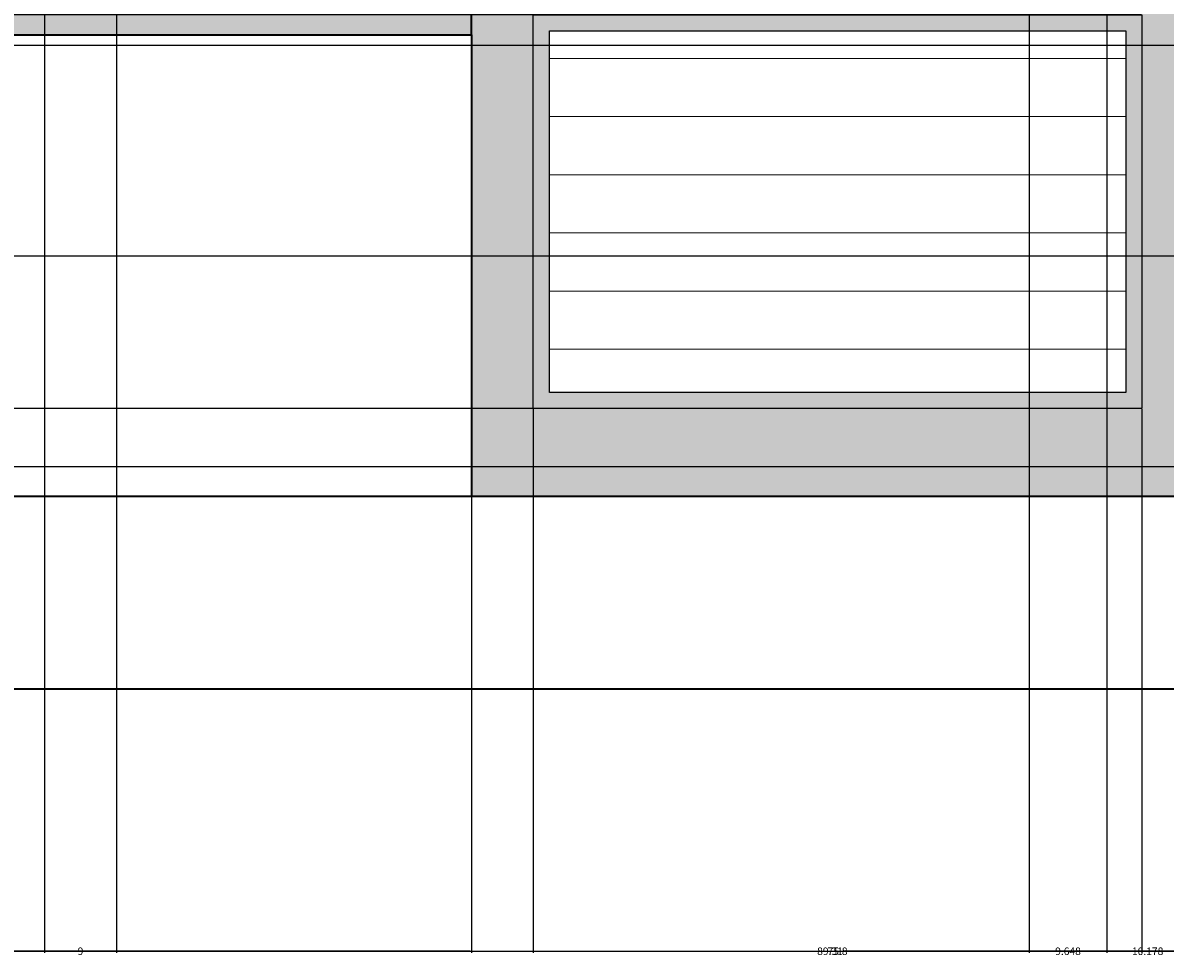
# Model space of a CAD drawing. Units: inches. Extents: x -5 to 714, y 84 to 644.
# Tile 3 of 20: x 124 to 266, y 84 to 200. Entities that reach past the tile are written whole.
import ezdxf

# ---------------------------------------------------------------- set-up
doc = ezdxf.new("R2010")
doc.units = ezdxf.units.IN
doc.header["$MEASUREMENT"] = 0
for name, color, linetype, lineweight in [('A-ANNO-DIMS', 2, 'Continuous', 18), ('A-ELEV', 7, 'Continuous', 35), ('A-ELEV-PATT', 8, 'Continuous', 13), ('A-GLAZ', 3, 'Continuous', 25)]:
    doc.layers.add(name, color=color, linetype=linetype, lineweight=lineweight)
doc.styles.get("Standard").update_dxf_attribs({"font": 'arial.ttf'})
doc.dimstyles.get("Standard").update_dxf_attribs({"dimtxt": 0.9375, "dimasz": 0.18, "dimexe": 0.18, "dimexo": 0.0625, "dimgap": 0.09, "dimtad": 0, "dimtih": 1, "dimtoh": 1, "dimdec": 4, "dimzin": 0, "dimdsep": 46, "dimlunit": 4, "dimtxsty": 'Standard', "dimcen": 0.09, "dimadec": 0, "dimazin": 0, "dimtfac": 1, "dimtdec": 4, "dimtofl": 0, "dimtmove": 0, "dimatfit": 3, "dimfxl": 1, "dimtolj": 1, "dimtzin": 0, "dimarcsym": 0})

# ---------------------------------------------------------------- blocks, each defined once
blk = doc.blocks.new('*D1')
at = {"layer": 'A-ANNO-DIMS', "color": 0, "lineweight": -2, "transparency": 16777216}
for p, q in [((30.14, 117.13), (30.14, 84.31)), ((679.78, 117.13), (679.78, 84.31)), ((30.32, 84.49), (353.29, 84.49)), ((679.6, 84.49), (356.64, 84.49))]:
    blk.add_line(p, q, dxfattribs=at)
at = {"layer": 'A-ANNO-DIMS', "color": 0, "transparency": 16777216}
for points in [[(30.32, 84.52), (30.32, 84.46), (30.14, 84.49)], [(679.6, 84.52), (679.6, 84.46), (679.78, 84.49)]]:
    blk.add_solid(points, dxfattribs=at)
at = {"layer": 'Defpoints', "color": 0, "transparency": 16777216}
for p in [(30.14, 117.19), (679.78, 117.19), (679.78, 84.49)]:
    blk.add_point(p, dxfattribs=at)
at = {"layer": 'A-ANNO-DIMS', "color": 0, "transparency": 16777216, "insert": (354.96, 84.49), "char_height": 0.938, "attachment_point": 5}
blk.add_mtext('\\A1;649.6', dxfattribs=at)
blk = doc.blocks.new('*D28')
at = {"layer": 'A-ANNO-DIMS', "color": 0, "lineweight": -2, "transparency": 16777216}
for p, q in [((126.73, 480.11), (126.73, 84.31)), ((135.73, 471.11), (135.73, 84.31)), ((126.91, 84.49), (130.83, 84.49)), ((135.55, 84.49), (131.63, 84.49))]:
    blk.add_line(p, q, dxfattribs=at)
at = {"layer": 'A-ANNO-DIMS', "color": 0, "transparency": 16777216}
for points in [[(126.91, 84.52), (126.91, 84.46), (126.73, 84.49)], [(135.55, 84.52), (135.55, 84.46), (135.73, 84.49)]]:
    blk.add_solid(points, dxfattribs=at)
at = {"layer": 'Defpoints', "color": 0, "transparency": 16777216}
for p in [(126.73, 480.17), (135.73, 471.17), (135.73, 84.49)]:
    blk.add_point(p, dxfattribs=at)
at = {"layer": 'A-ANNO-DIMS', "color": 0, "transparency": 16777216, "insert": (131.23, 84.49), "char_height": 0.938, "attachment_point": 5}
blk.add_mtext('\\A1;9', dxfattribs=at)
blk = doc.blocks.new('*D29')
at = {"layer": 'A-ANNO-DIMS', "color": 0, "lineweight": -2, "transparency": 16777216}
for p, q in [((135.73, 471.11), (135.73, 84.31)), ((429.51, 471.11), (429.51, 84.31)), ((135.91, 84.49), (280.94, 84.49)), ((429.33, 84.49), (284.3, 84.49))]:
    blk.add_line(p, q, dxfattribs=at)
at = {"layer": 'A-ANNO-DIMS', "color": 0, "transparency": 16777216}
for points in [[(135.91, 84.52), (135.91, 84.46), (135.73, 84.49)], [(429.33, 84.52), (429.33, 84.46), (429.51, 84.49)]]:
    blk.add_solid(points, dxfattribs=at)
at = {"layer": 'Defpoints', "color": 0, "transparency": 16777216}
for p in [(135.73, 471.17), (429.51, 471.17), (429.51, 84.49)]:
    blk.add_point(p, dxfattribs=at)
at = {"layer": 'A-ANNO-DIMS', "color": 0, "transparency": 16777216, "insert": (282.62, 84.49), "char_height": 0.938, "attachment_point": 5}
blk.add_mtext('\\A1;293.8', dxfattribs=at)
blk = doc.blocks.new('*D52')
at = {"layer": 'A-ANNO-DIMS', "color": 0, "lineweight": -2, "transparency": 16777216}
for p, q in [((249.42, 345.13), (249.42, 84.31)), ((259.07, 345.13), (259.07, 84.31)), ((249.6, 84.49), (252.57, 84.49)), ((258.89, 84.49), (255.92, 84.49))]:
    blk.add_line(p, q, dxfattribs=at)
at = {"layer": 'A-ANNO-DIMS', "color": 0, "transparency": 16777216}
for points in [[(249.6, 84.52), (249.6, 84.46), (249.42, 84.49)], [(258.89, 84.52), (258.89, 84.46), (259.07, 84.49)]]:
    blk.add_solid(points, dxfattribs=at)
at = {"layer": 'Defpoints', "color": 0, "transparency": 16777216}
for p in [(249.42, 345.19), (259.07, 345.19), (259.07, 84.49)]:
    blk.add_point(p, dxfattribs=at)
at = {"layer": 'A-ANNO-DIMS', "color": 0, "transparency": 16777216, "insert": (254.24, 84.49), "char_height": 0.938, "attachment_point": 5}
blk.add_mtext('\\A1;9.648', dxfattribs=at)
blk = doc.blocks.new('*D53')
at = {"layer": 'A-ANNO-DIMS', "color": 0, "lineweight": -2, "transparency": 16777216}
for p, q in [((259.07, 315.03), (259.07, 84.31)), ((269.24, 306.57), (269.24, 84.31)), ((259.25, 84.49), (262.16, 84.49)), ((269.06, 84.49), (266.15, 84.49))]:
    blk.add_line(p, q, dxfattribs=at)
at = {"layer": 'A-ANNO-DIMS', "color": 0, "transparency": 16777216}
for points in [[(259.25, 84.52), (259.25, 84.46), (259.07, 84.49)], [(269.06, 84.52), (269.06, 84.46), (269.24, 84.49)]]:
    blk.add_solid(points, dxfattribs=at)
at = {"layer": 'Defpoints', "color": 0, "transparency": 16777216}
for p in [(259.07, 315.1), (269.24, 306.63), (269.24, 84.49)]:
    blk.add_point(p, dxfattribs=at)
at = {"layer": 'A-ANNO-DIMS', "color": 0, "transparency": 16777216, "insert": (264.16, 84.49), "char_height": 0.938, "attachment_point": 5}
blk.add_mtext('\\A1;10.178', dxfattribs=at)
blk = doc.blocks.new('*D65')
at = {"layer": 'A-ANNO-DIMS', "color": 0, "lineweight": -2, "transparency": 16777216}
for p, q in [((325.77, 266), (-2.74, 266)), ((-2.56, 265.82), (-2.56, 219.13)), ((-2.56, 171.3), (-2.56, 217.99)), ((325.77, 171.12), (-2.74, 171.12))]:
    blk.add_line(p, q, dxfattribs=at)
at = {"layer": 'A-ANNO-DIMS', "color": 0, "transparency": 16777216}
for points in [[(-2.59, 265.82), (-2.53, 265.82), (-2.56, 266)], [(-2.59, 171.3), (-2.53, 171.3), (-2.56, 171.12)]]:
    blk.add_solid(points, dxfattribs=at)
at = {"layer": 'Defpoints', "color": 0, "transparency": 16777216}
for p in [(-2.56, 266), (325.83, 266), (325.83, 171.12)]:
    blk.add_point(p, dxfattribs=at)
at = {"layer": 'A-ANNO-DIMS', "color": 0, "transparency": 16777216, "insert": (-2.56, 218.56), "char_height": 0.938, "attachment_point": 5}
blk.add_mtext('\\A1;94.88', dxfattribs=at)
blk = doc.blocks.new('*D73')
at = {"layer": 'A-ANNO-DIMS', "color": 0, "lineweight": -2, "transparency": 16777216}
for p, q in [((30.14, 141.13), (30.14, 84.31)), ((179.93, 141.13), (179.93, 84.31)), ((30.32, 84.49), (103.41, 84.49)), ((179.75, 84.49), (106.67, 84.49))]:
    blk.add_line(p, q, dxfattribs=at)
at = {"layer": 'A-ANNO-DIMS', "color": 0, "transparency": 16777216}
for points in [[(30.32, 84.52), (30.32, 84.46), (30.14, 84.49)], [(179.75, 84.52), (179.75, 84.46), (179.93, 84.49)]]:
    blk.add_solid(points, dxfattribs=at)
at = {"layer": 'Defpoints', "color": 0, "transparency": 16777216}
for p in [(30.14, 141.19), (179.93, 141.19), (179.93, 84.49)]:
    blk.add_point(p, dxfattribs=at)
at = {"layer": 'A-ANNO-DIMS', "color": 0, "transparency": 16777216, "insert": (105.04, 84.49), "char_height": 0.938, "attachment_point": 5}
blk.add_mtext('\\A1;149.8', dxfattribs=at)
blk = doc.blocks.new('*D74')
at = {"layer": 'A-ANNO-DIMS', "color": 0, "lineweight": -2, "transparency": 16777216}
for p, q in [((179.93, 141.13), (179.93, 84.31)), ((269.24, 141.13), (269.24, 84.31)), ((180.11, 84.49), (223.01, 84.49)), ((269.06, 84.49), (226.17, 84.49))]:
    blk.add_line(p, q, dxfattribs=at)
at = {"layer": 'A-ANNO-DIMS', "color": 0, "transparency": 16777216}
for points in [[(180.11, 84.52), (180.11, 84.46), (179.93, 84.49)], [(269.06, 84.52), (269.06, 84.46), (269.24, 84.49)]]:
    blk.add_solid(points, dxfattribs=at)
at = {"layer": 'Defpoints', "color": 0, "transparency": 16777216}
for p in [(179.93, 141.19), (269.24, 141.19), (269.24, 84.49)]:
    blk.add_point(p, dxfattribs=at)
at = {"layer": 'A-ANNO-DIMS', "color": 0, "transparency": 16777216, "insert": (224.59, 84.49), "char_height": 0.938, "attachment_point": 5}
blk.add_mtext('\\A1;89.31', dxfattribs=at)
blk = doc.blocks.new('*D81')
at = {"layer": 'A-ANNO-DIMS', "color": 0, "lineweight": -2, "transparency": 16777216}
for p, q in [((187.63, 152.06), (187.63, 84.31)), ((263.43, 152.06), (263.43, 84.31)), ((187.81, 84.49), (224.23, 84.49)), ((263.25, 84.49), (226.84, 84.49))]:
    blk.add_line(p, q, dxfattribs=at)
at = {"layer": 'A-ANNO-DIMS', "color": 0, "transparency": 16777216}
for points in [[(187.81, 84.52), (187.81, 84.46), (187.63, 84.49)], [(263.25, 84.52), (263.25, 84.46), (263.43, 84.49)]]:
    blk.add_solid(points, dxfattribs=at)
at = {"layer": 'Defpoints', "color": 0, "transparency": 16777216}
for p in [(187.63, 152.12), (263.43, 152.12), (263.43, 84.49)]:
    blk.add_point(p, dxfattribs=at)
at = {"layer": 'A-ANNO-DIMS', "color": 0, "transparency": 16777216, "insert": (225.53, 84.49), "char_height": 0.938, "attachment_point": 5}
blk.add_mtext('\\A1;75.8', dxfattribs=at)
blk = doc.blocks.new('*D82')
at = {"layer": 'A-ANNO-DIMS', "color": 0, "lineweight": -2, "transparency": 16777216}
for p, q in [((263.37, 201.19), (-2.74, 201.19)), ((-2.56, 201.01), (-2.56, 177.22)), ((-2.56, 152.3), (-2.56, 176.09)), ((263.37, 152.12), (-2.74, 152.12))]:
    blk.add_line(p, q, dxfattribs=at)
at = {"layer": 'A-ANNO-DIMS', "color": 0, "transparency": 16777216}
for points in [[(-2.59, 201.01), (-2.53, 201.01), (-2.56, 201.19)], [(-2.59, 152.3), (-2.53, 152.3), (-2.56, 152.12)]]:
    blk.add_solid(points, dxfattribs=at)
at = {"layer": 'Defpoints', "color": 0, "transparency": 16777216}
for p in [(-2.56, 201.19), (263.43, 201.19), (263.43, 152.12)]:
    blk.add_point(p, dxfattribs=at)
at = {"layer": 'A-ANNO-DIMS', "color": 0, "transparency": 16777216, "insert": (-2.56, 176.66), "char_height": 0.938, "attachment_point": 5}
blk.add_mtext('\\A1;49.08', dxfattribs=at)
blk = doc.blocks.new('*D87')
at = {"layer": 'A-ANNO-DIMS', "color": 0, "lineweight": -2, "transparency": 16777216}
for p, q in [((306.9, 197.38), (-2.74, 197.38)), ((-2.56, 197.2), (-2.56, 171.69)), ((-2.56, 145.04), (-2.56, 170.55)), ((306.9, 144.86), (-2.74, 144.86))]:
    blk.add_line(p, q, dxfattribs=at)
at = {"layer": 'A-ANNO-DIMS', "color": 0, "transparency": 16777216}
for points in [[(-2.59, 197.2), (-2.53, 197.2), (-2.56, 197.38)], [(-2.59, 145.04), (-2.53, 145.04), (-2.56, 144.86)]]:
    blk.add_solid(points, dxfattribs=at)
at = {"layer": 'Defpoints', "color": 0, "transparency": 16777216}
for p in [(-2.56, 197.38), (306.96, 197.38), (306.96, 144.86)]:
    blk.add_point(p, dxfattribs=at)
at = {"layer": 'A-ANNO-DIMS', "color": 0, "transparency": 16777216, "insert": (-2.56, 171.12), "char_height": 0.938, "attachment_point": 5}
blk.add_mtext('\\A1;52.51', dxfattribs=at)
blk = doc.blocks.new('*D89')
at = {"layer": 'A-ANNO-DIMS', "color": 0, "lineweight": -2, "transparency": 16777216}
for p, q in [((541.31, 197.38), (-2.74, 197.38)), ((-2.56, 197.2), (-2.56, 171.69)), ((-2.56, 145.04), (-2.56, 170.55)), ((541.31, 144.86), (-2.74, 144.86))]:
    blk.add_line(p, q, dxfattribs=at)
at = {"layer": 'A-ANNO-DIMS', "color": 0, "transparency": 16777216}
for points in [[(-2.59, 197.2), (-2.53, 197.2), (-2.56, 197.38)], [(-2.59, 145.04), (-2.53, 145.04), (-2.56, 144.86)]]:
    blk.add_solid(points, dxfattribs=at)
at = {"layer": 'Defpoints', "color": 0, "transparency": 16777216}
for p in [(-2.56, 197.38), (541.38, 197.38), (541.38, 144.86)]:
    blk.add_point(p, dxfattribs=at)
at = {"layer": 'A-ANNO-DIMS', "color": 0, "transparency": 16777216, "insert": (-2.56, 171.12), "char_height": 0.938, "attachment_point": 5}
blk.add_mtext('\\A1;52.51', dxfattribs=at)

msp = doc.modelspace()

# ---------------------------------------------------------------- hatches: boundary and pattern name
at = {"layer": 'A-ELEV-PATT', "transparency": 33554687}
h = msp.add_hatch(color=256, dxfattribs=at)
h.dxf.hatch_style = 1
h.paths.add_polyline_path([(188.3677, 525.1928), (67.9893, 525.1928), (67.9893, 489.1928), (67.9893, 345.1928), (126.7303, 345.1928), (126.7303, 480.1709), (229.3575, 480.1709), (229.3575, 525.1928), (212.6043, 525.1928), (212.6043, 482.7164), (211.0019, 482.7164), (211.0019, 525.1928), (207.6919, 525.1928), (199.9852, 525.1928), (199.9852, 482.7164), (198.3828, 482.7164), (198.3828, 525.1928), (189.9701, 525.1928), (189.9701, 482.7164), (188.3677, 482.7164)])
h.paths.add_polyline_path([(121.3589, 336.2066), (75.5048, 336.2066), (75.5048, 319.345), (121.3589, 319.345)])
h.paths.add_polyline_path([(121.3589, 319.345), (75.5048, 319.345), (75.5048, 302.3045), (121.3589, 302.3045)])
h.paths.add_polyline_path([(121.3589, 302.3045), (75.5048, 302.3045), (75.5048, 282.8561), (121.3589, 282.8561)])
h.paths.add_polyline_path([(121.3589, 282.8561), (75.5048, 282.8561), (75.5048, 261.5556), (121.3589, 261.5556)])
h.paths.add_polyline_path([(121.3589, 261.5556), (75.5048, 261.5556), (75.5048, 243.7009), (121.3589, 243.7009)])
h.paths.add_polyline_path([(121.3589, 243.7009), (75.5048, 243.7009), (75.5048, 223.5117), (121.3589, 223.5117)])
h.paths.add_polyline_path([(121.3589, 223.5117), (75.5048, 223.5117), (75.5048, 212.5836), (121.3589, 212.5836)])
h.paths.add_polyline_path([(121.3589, 212.5836), (75.5048, 212.5836), (75.5048, 201.1928), (121.3589, 201.1928)])
h.paths.add_polyline_path([(179.9335, 201.1928), (30.1395, 201.1928), (30.1395, 198.7054), (179.9335, 198.7054)])
h.paths.add_polyline_path([(187.6349, 201.1928), (179.9335, 201.1928), (179.9335, 198.7054), (179.9335, 141.1928), (269.2446, 141.1928), (269.2446, 201.1928), (263.4349, 201.1928), (263.4349, 152.1176), (187.6349, 152.1176)])
h.paths.add_polyline_path([(269.2446, 277.0513), (269.2446, 287.501), (269.2446, 306.6286), (578.0915, 306.6286), (578.0915, 201.1928), (593.428, 201.1928), (593.428, 315.0968), (584.4202, 315.0968), (259.0665, 315.0968), (259.0665, 201.1928), (263.4349, 201.1928), (269.2446, 201.1928)])
h = msp.add_hatch(dxfattribs=at)
h.set_pattern_fill('ANSI31', color=256, scale=58, angle=135)
h.paths.add_polyline_path([(249.4181, 345.1928), (237.2654, 345.1928), (200.7361, 345.1928), (200.7361, 201.1928), (249.4181, 201.1928)])
h.paths.add_polyline_path([(261.4349, 199.1928), (189.6349, 199.1928), (189.6349, 154.1176), (261.4349, 154.1176)])
h.paths.add_polyline_path([(415.8092, 525.1928), (366.2809, 525.1928), (366.2809, 480.1709), (415.8092, 480.1709)])
h = msp.add_hatch(color=256, dxfattribs=at)
h.dxf.hatch_style = 1
h.paths.add_polyline_path([(263.4349, 201.1928), (187.6349, 201.1928), (187.6349, 152.1176), (263.4349, 152.1176)])
h.paths.add_polyline_path([(189.6349, 199.1928), (261.4349, 199.1928), (261.4349, 154.1176), (189.6349, 154.1176)], flags=16)

# ---------------------------------------------------------------- linework, layer by layer
at = {"layer": 'A-ELEV'}
for p, q in [((179.9335, 198.7054), (179.9335, 201.1928)), ((30.1395, 198.7054), (179.9335, 198.7054)), ((179.9335, 198.7054), (179.9335, 141.1928)), ((30.1395, 141.1928), (548.9353, 141.1928)), ((30.1395, 117.1928), (548.9353, 117.1928))]:
    msp.add_line(p, q, dxfattribs=at)
at = {"layer": 'A-GLAZ'}
for points in [[(187.6349, 201.1928), (263.4349, 201.1928), (263.4349, 152.1176), (187.6349, 152.1176)], [(189.6349, 199.1928), (261.4349, 199.1928), (261.4349, 154.1176), (189.6349, 154.1176)]]:
    msp.add_lwpolyline(points, close=True, dxfattribs=at)

# ---------------------------------------------------------------- dimensions: what is measured, and where the dimension line sits
at = {"layer": 'A-ANNO-DIMS'}
for base, p1, p2, override, picture, middle in [((135.7303, 84.4928), (126.7303, 480.1709), (135.7303, 471.1709), {"dimdec": 0, "dimlfac": 1, "dimrnd": 0, "dimzin": 0, "dimdsep": 46, "dimlunit": 2}, '*D28', (131.2303, 84.4928)), ((429.5094, 84.4928), (135.7303, 471.1709), (429.5094, 471.1709), {"dimdec": 1, "dimlfac": 1, "dimrnd": 0, "dimzin": 0, "dimdsep": 46, "dimlunit": 2}, '*D29', (282.6198, 84.4928)), ((259.0665, 84.4928), (249.4181, 345.1928), (259.0665, 345.1928), {"dimdec": 3, "dimlfac": 1, "dimrnd": 0, "dimzin": 0, "dimdsep": 46, "dimlunit": 2}, '*D52', (254.2423, 84.4928)), ((269.2446, 84.4928), (259.0665, 315.0968), (269.2446, 306.6286), {"dimdec": 3, "dimlfac": 1, "dimrnd": 0, "dimzin": 0, "dimdsep": 46, "dimlunit": 2}, '*D53', (264.1555, 84.4928)), ((263.4349, 84.4928), (187.6349, 152.1176), (263.4349, 152.1176), {"dimdec": 1, "dimlfac": 1, "dimrnd": 0, "dimzin": 0, "dimdsep": 46, "dimlunit": 2}, '*D81', (225.5349, 84.4928)), ((179.9335, 84.4928), (30.1395, 141.1928), (179.9335, 141.1928), {"dimdec": 1, "dimlfac": 1, "dimrnd": 0, "dimzin": 0, "dimdsep": 46, "dimlunit": 2}, '*D73', (105.0365, 84.4928)), ((269.2446, 84.4928), (179.9335, 141.1928), (269.2446, 141.1928), {"dimdec": 2, "dimlfac": 1, "dimrnd": 0, "dimzin": 0, "dimdsep": 46, "dimlunit": 2}, '*D74', (224.5891, 84.4928)), ((679.7826, 84.4928), (30.1395, 117.1928), (679.7826, 117.1928), {"dimdec": 1, "dimlfac": 1, "dimrnd": 0, "dimzin": 0, "dimdsep": 46, "dimlunit": 2}, '*D1', (354.9611, 84.4928))]:
    dim = msp.add_linear_dim(base=base, p1=p1, p2=p2, dimstyle='Standard', override=override, dxfattribs=at)
    dim.commit()
    dim.dimension.update_dxf_attribs({"geometry": picture, "text_midpoint": middle})
for base, p1, p2, picture, middle in [((-2.5605, 266.0021), (325.8305, 171.1197), (325.8305, 266.0021), '*D65', (-2.5605, 218.5609)), ((-2.5605, 201.1928), (263.4349, 152.1176), (263.4349, 201.1928), '*D82', (-2.5605, 176.6552)), ((-2.5605, 197.3754), (306.958, 144.8639), (306.958, 197.3754), '*D87', (-2.5605, 171.1197)), ((-2.5605, 197.3754), (541.3773, 144.8639), (541.3773, 197.3754), '*D89', (-2.5605, 171.1197))]:
    dim = msp.add_linear_dim(base=base, p1=p1, p2=p2, angle=90, dimstyle='Standard', override={"dimdec": 2, "dimlfac": 1, "dimrnd": 0, "dimzin": 0, "dimdsep": 46, "dimlunit": 2}, dxfattribs=at)
    dim.commit()
    dim.dimension.update_dxf_attribs({"geometry": picture, "text_midpoint": middle})

doc.saveas('drawing.dxf')
